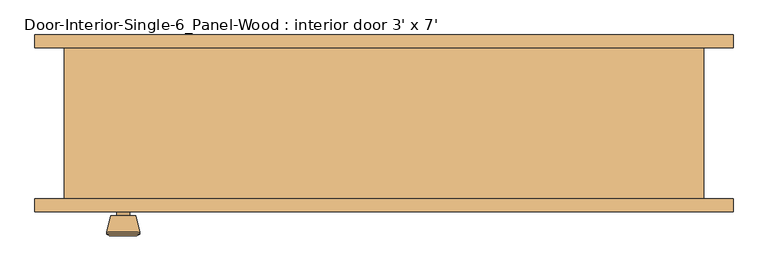
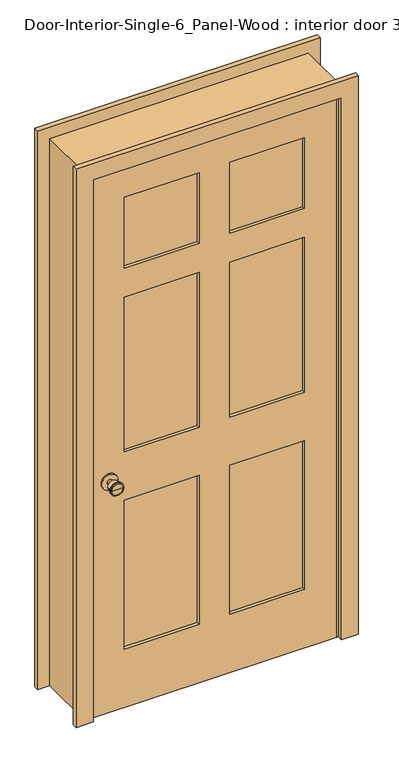
"""IFC4 building model written with IfcOpenShell, lengths in millimetres: door geometry, Door-Interior-Single-6_Panel-Wood : interior door 3' x 7'."""

from ifc_helpers import new_model, si_unit, point, frame, frame_2d, origin, place, context, project, spatial, polyline, circle_curve, trimmed, segment, composite_curve, outline, extrude, faceted_brep, source, transform, mapped, element, save
from ifc_brep_helpers import plane_surface, cylinder_surface, revolved_surface, advanced_brep


def door_interior_single_6_panel_wood_interior_door_3_x_7_c5239341(model_context):
    return source(origin(), model_context, "Body", "SolidModel", [
        advanced_brep(
        [(-393.7, -70.2, 914.4), (-403.7, -70.2, 914.4), (-383.7, -70.2, 914.4), (-373.2241324, -21.2, 914.4), (-414.1758676, -21.2, 914.4), (-393.7, -21.2, 914.4), (-368.7, -23.0278681, 914.4), (-418.7, -23.0278681, 914.4), (-368.7, -26.4915463, 914.4), (-418.7, -26.4915463, 914.4), (-375.063764, -51.2, 914.4), (-412.336236, -51.2, 914.4), (-383.7, -51.2, 914.4), (-403.7, -51.2, 914.4)],
        [
            (0, 1),
            (1, 2, circle_curve(frame((-393.7, -70.2, 914.4), z_axis=(0.0, -1.0, 0.0), x_axis=(-1.0, 0.0, 0.0)), 10.0)),
            (2, 0),
            (2, 1, circle_curve(frame((-393.7, -70.2, 914.4), z_axis=(0.0, -1.0, 0.0), x_axis=(-1.0, 0.0, 0.0)), 10.0)),
            (3, 4, circle_curve(frame((-393.7, -21.2, 914.4), z_axis=(0.0, 1.0, 0.0), x_axis=(-1.0, 0.0, 0.0)), 20.4758676)),
            (4, 5),
            (5, 3),
            (4, 3, circle_curve(frame((-393.7, -21.2, 914.4), z_axis=(0.0, 1.0, 0.0), x_axis=(-1.0, 0.0, 0.0)), 20.4758676)),
            (6, 7, circle_curve(frame((-393.7, -23.0278681, 914.4), z_axis=(0.0, 1.0, 0.0), x_axis=(-1.0, 0.0, 0.0)), 25.0)),
            (7, 4),
            (3, 6),
            (7, 6, circle_curve(frame((-393.7, -23.0278681, 914.4), z_axis=(0.0, 1.0, 0.0), x_axis=(-1.0, 0.0, 0.0)), 25.0)),
            (8, 9, circle_curve(frame((-393.7, -26.4915463, 914.4), z_axis=(0.0, 1.0, 0.0), x_axis=(-1.0, 0.0, 0.0)), 25.0)),
            (9, 7),
            (6, 8),
            (9, 8, circle_curve(frame((-393.7, -26.4915463, 914.4), z_axis=(0.0, 1.0, 0.0), x_axis=(-1.0, 0.0, 0.0)), 25.0)),
            (10, 11, circle_curve(frame((-393.7, -51.2, 914.4), z_axis=(0.0, 1.0, 0.0), x_axis=(-1.0, 0.0, 0.0)), 18.636236)),
            (11, 9),
            (8, 10),
            (11, 10, circle_curve(frame((-393.7, -51.2, 914.4), z_axis=(0.0, 1.0, 0.0), x_axis=(-1.0, 0.0, 0.0)), 18.636236)),
            (12, 13, circle_curve(frame((-393.7, -51.2, 914.4), z_axis=(0.0, 1.0, 0.0), x_axis=(-1.0, 0.0, 0.0)), 10.0)),
            (13, 11),
            (10, 12),
            (13, 12, circle_curve(frame((-393.7, -51.2, 914.4), z_axis=(0.0, 1.0, 0.0), x_axis=(-1.0, 0.0, 0.0)), 10.0)),
            (1, 13),
            (12, 2),
        ],
        [
            plane_surface(frame((-393.7, -70.2, 914.4), z_axis=(0.0, -1.0, 0.0), x_axis=(-1.0, 0.0, 0.0))),
            plane_surface(frame((-393.7, -21.2, 914.4), z_axis=(0.0, 1.0, 0.0), x_axis=(-1.0, 0.0, 0.0))),
            revolved_surface(polyline([(-414.1758676, -21.2, 914.4), (-418.7, -23.0278681, 914.4)]), (-393.7, -70.2, 914.4), (0.0, -1.0, 0.0)),
            cylinder_surface(frame((-393.7, -70.2, 914.4), z_axis=(0.0, -1.0, 0.0), x_axis=(-1.0, 0.0, 0.0)), 25.0),
            revolved_surface(polyline([(-418.7, -26.4915463, 914.4), (-412.336236, -51.2, 914.4)]), (-393.7, -70.2, 914.4), (0.0, -1.0, 0.0)),
            plane_surface(frame((-393.7, -51.2, 914.4), z_axis=(0.0, -1.0, 0.0), x_axis=(-1.0, 0.0, 0.0))),
            cylinder_surface(frame((-393.7, -70.2, 914.4), z_axis=(0.0, -1.0, 0.0), x_axis=(-1.0, 0.0, 0.0)), 10.0),
        ],
        [
            (0, [[1, 2, 3]]),
            (0, [[-3, 4, -1]]),
            (1, [[5, 6, 7]]),
            (1, [[8, -7, -6]]),
            (2, [[9, 10, -5, 11]]),
            (2, [[12, -11, -8, -10]]),
            (3, [[13, 14, -9, 15]]),
            (3, [[16, -15, -12, -14]]),
            (4, [[17, 18, -13, 19]]),
            (4, [[20, -19, -16, -18]]),
            (5, [[21, 22, -17, 23]]),
            (5, [[24, -23, -20, -22]]),
            (6, [[-2, 25, -21, 26]]),
            (6, [[-4, -26, -24, -25]]),
        ],
    ),
        extrude(outline(composite_curve([segment(trimmed(circle_curve(frame_2d((914.4, -393.7)), 30.0), [point((914.4, -423.7))], [point((914.4, -363.7))], False, "CARTESIAN"), True, "CONTINUOUS"), segment(trimmed(circle_curve(frame_2d((914.4, -393.7)), 30.0), [point((914.4, -363.7))], [point((914.4, -423.7))], False, "CARTESIAN"), True, "CONTINUOUS")], self_intersect=False)), frame((0.0, -76.2, 0.0), z_axis=(0.0, 1.0, 0.0), x_axis=(0.0, 0.0, 1.0)), (0.0, 0.0, 1.0), 6.0),
        advanced_brep(
        [(-393.7, -117.125, 914.4), (-383.7, -117.125, 914.4), (-403.7, -117.125, 914.4), (-373.2241324, -166.125, 914.4), (-393.7, -166.125, 914.4), (-414.1758676, -166.125, 914.4), (-368.7, -164.2971319, 914.4), (-418.7, -164.2971319, 914.4), (-368.7, -160.8334537, 914.4), (-418.7, -160.8334537, 914.4), (-375.063764, -136.125, 914.4), (-412.336236, -136.125, 914.4), (-383.7, -136.125, 914.4), (-403.7, -136.125, 914.4)],
        [
            (0, 1),
            (1, 2, circle_curve(frame((-393.7, -117.125, 914.4), z_axis=(0.0, 1.0, 0.0), x_axis=(-1.0, 0.0, 0.0)), 10.0)),
            (2, 0),
            (2, 1, circle_curve(frame((-393.7, -117.125, 914.4), z_axis=(0.0, 1.0, 0.0), x_axis=(-1.0, 0.0, 0.0)), 10.0)),
            (3, 4),
            (4, 5),
            (5, 3, circle_curve(frame((-393.7, -166.125, 914.4), z_axis=(0.0, -1.0, 0.0), x_axis=(-1.0, 0.0, 0.0)), 20.4758676)),
            (3, 5, circle_curve(frame((-393.7, -166.125, 914.4), z_axis=(0.0, -1.0, 0.0), x_axis=(-1.0, 0.0, 0.0)), 20.4758676)),
            (6, 3),
            (5, 7),
            (7, 6, circle_curve(frame((-393.7, -164.2971319, 914.4), z_axis=(0.0, -1.0, 0.0), x_axis=(-1.0, 0.0, 0.0)), 25.0)),
            (6, 7, circle_curve(frame((-393.7, -164.2971319, 914.4), z_axis=(0.0, -1.0, 0.0), x_axis=(-1.0, 0.0, 0.0)), 25.0)),
            (8, 6),
            (7, 9),
            (9, 8, circle_curve(frame((-393.7, -160.8334537, 914.4), z_axis=(0.0, -1.0, 0.0), x_axis=(-1.0, 0.0, 0.0)), 25.0)),
            (8, 9, circle_curve(frame((-393.7, -160.8334537, 914.4), z_axis=(0.0, -1.0, 0.0), x_axis=(-1.0, 0.0, 0.0)), 25.0)),
            (10, 8),
            (9, 11),
            (11, 10, circle_curve(frame((-393.7, -136.125, 914.4), z_axis=(0.0, -1.0, 0.0), x_axis=(-1.0, 0.0, 0.0)), 18.636236)),
            (10, 11, circle_curve(frame((-393.7, -136.125, 914.4), z_axis=(0.0, -1.0, 0.0), x_axis=(-1.0, 0.0, 0.0)), 18.636236)),
            (12, 10),
            (11, 13),
            (13, 12, circle_curve(frame((-393.7, -136.125, 914.4), z_axis=(0.0, -1.0, 0.0), x_axis=(-1.0, 0.0, 0.0)), 10.0)),
            (12, 13, circle_curve(frame((-393.7, -136.125, 914.4), z_axis=(0.0, -1.0, 0.0), x_axis=(-1.0, 0.0, 0.0)), 10.0)),
            (1, 12),
            (13, 2),
        ],
        [
            plane_surface(frame((-393.7, -117.125, 914.4), z_axis=(0.0, 1.0, 0.0), x_axis=(-1.0, 0.0, 0.0))),
            plane_surface(frame((-393.7, -166.125, 914.4), z_axis=(0.0, -1.0, 0.0), x_axis=(-1.0, 0.0, 0.0))),
            revolved_surface(polyline([(-414.1758676, -166.125, 914.4), (-418.7, -164.2971319, 914.4)]), (-393.7, -117.125, 914.4), (0.0, 1.0, 0.0)),
            cylinder_surface(frame((-393.7, -117.125, 914.4), z_axis=(0.0, 1.0, 0.0), x_axis=(-1.0, 0.0, 0.0)), 25.0),
            revolved_surface(polyline([(-418.7, -160.8334537, 914.4), (-412.336236, -136.125, 914.4)]), (-393.7, -117.125, 914.4), (0.0, 1.0, 0.0)),
            plane_surface(frame((-393.7, -136.125, 914.4), z_axis=(0.0, 1.0, 0.0), x_axis=(-1.0, 0.0, 0.0))),
            cylinder_surface(frame((-393.7, -117.125, 914.4), z_axis=(0.0, 1.0, 0.0), x_axis=(-1.0, 0.0, 0.0)), 10.0),
        ],
        [
            (0, [[1, 2, 3]]),
            (0, [[-3, 4, -1]]),
            (1, [[5, 6, 7]]),
            (1, [[-6, -5, 8]]),
            (2, [[9, -7, 10, 11]]),
            (2, [[-10, -8, -9, 12]]),
            (3, [[13, -11, 14, 15]]),
            (3, [[-14, -12, -13, 16]]),
            (4, [[17, -15, 18, 19]]),
            (4, [[-18, -16, -17, 20]]),
            (5, [[21, -19, 22, 23]]),
            (5, [[-22, -20, -21, 24]]),
            (6, [[25, -23, 26, -2]]),
            (6, [[-26, -24, -25, -4]]),
        ],
    ),
        extrude(outline(composite_curve([segment(trimmed(circle_curve(frame_2d((914.4, -393.7)), 30.0), [point((914.4, -423.7))], [point((914.4, -363.7))], False, "CARTESIAN"), True, "CONTINUOUS"), segment(trimmed(circle_curve(frame_2d((914.4, -393.7)), 30.0), [point((914.4, -363.7))], [point((914.4, -423.7))], False, "CARTESIAN"), True, "CONTINUOUS")], self_intersect=False)), frame((0.0, -117.125, 0.0), z_axis=(0.0, 1.0, 0.0), x_axis=(0.0, 0.0, 1.0)), (0.0, 0.0, 1.0), 6.0),
        faceted_brep([(482.6, -111.125, 0.0), (457.2, -111.125, 0.0), (457.2, -76.2, 0.0), (444.5, -76.2, 0.0), (444.5, -41.275, 0.0), (457.2, -41.275, 0.0), (457.2, 117.475, 0.0), (482.6, 117.475, 0.0), (482.6, 117.475, 2159.0), (482.6, -111.125, 2159.0), (457.2, 117.475, 2133.6), (-457.2, 117.475, 2133.6), (-457.2, 117.475, 0.0), (-482.6, 117.475, 0.0), (-482.6, 117.475, 2159.0), (457.2, -41.275, 2133.6), (444.5, -41.275, 2120.9), (-444.5, -41.275, 2120.9), (-444.5, -41.275, 0.0), (-457.2, -41.275, 0.0), (-457.2, -41.275, 2133.6), (444.5, -76.2, 2120.9), (457.2, -76.2, 2133.6), (-457.2, -76.2, 2133.6), (-457.2, -76.2, 0.0), (-444.5, -76.2, 0.0), (-444.5, -76.2, 2120.9), (457.2, -111.125, 2133.6), (-482.6, -111.125, 2159.0), (-482.6, -111.125, 0.0), (-457.2, -111.125, 0.0), (-457.2, -111.125, 2133.6)], [[[0, 1, 2, 3, 4, 5, 6, 7]], [[7, 8, 9, 0]], [[6, 10, 11, 12, 13, 14, 8, 7]], [[5, 15, 10, 6]], [[4, 16, 17, 18, 19, 20, 15, 5]], [[3, 21, 16, 4]], [[2, 22, 23, 24, 25, 26, 21, 3]], [[1, 27, 22, 2]], [[0, 9, 28, 29, 30, 31, 27, 1]], [[8, 14, 28, 9]], [[15, 20, 11, 10]], [[21, 26, 17, 16]], [[27, 31, 23, 22]], [[29, 13, 12, 19, 18, 25, 24, 30]], [[14, 13, 29, 28]], [[20, 19, 12, 11]], [[26, 25, 18, 17]], [[31, 30, 24, 23]]]),
        extrude(outline(polyline([(2133.6, -457.2), (0.0, -457.2), (0.0, 457.2), (2133.6, 457.2), (2133.6, -457.2)]), holes=[polyline([(2014.5375, 57.15), (2014.5375, 336.55), (1735.1375, 336.55), (1735.1375, 57.15), (2014.5375, 57.15)]), polyline([(1620.8375, 336.55), (1009.65, 336.55), (1009.65, 57.15), (1620.8375, 57.15), (1620.8375, 336.55)]), polyline([(1009.65, -57.15), (1009.65, -336.55), (1620.8375, -336.55), (1620.8375, -57.15), (1009.65, -57.15)]), polyline([(1735.1375, -336.55), (2014.5375, -336.55), (2014.5375, -57.15), (1735.1375, -57.15), (1735.1375, -336.55)]), polyline([(819.15, 57.15), (819.15, 336.55), (231.775, 336.55), (231.775, 57.15), (819.15, 57.15)]), polyline([(231.775, -57.15), (231.775, -336.55), (819.15, -336.55), (819.15, -57.15), (231.775, -57.15)])]), frame((0.0, -111.125, 0.0), z_axis=(0.0, 1.0, 0.0), x_axis=(0.0, 0.0, 1.0)), (0.0, 0.0, 1.0), 34.925),
        extrude(outline(polyline([(336.55, -87.8416667), (336.55, -99.4833333), (57.15, -99.4833333), (57.15, -87.8416667), (336.55, -87.8416667)])), frame((0.0, 0.0, 1735.1375), z_axis=(0.0, 0.0, 1.0), x_axis=(1.0, 0.0, 0.0)), (0.0, 0.0, 1.0), 279.4),
        extrude(outline(polyline([(336.55, -87.8416667), (336.55, -99.4833333), (57.15, -99.4833333), (57.15, -87.8416667), (336.55, -87.8416667)])), frame((0.0, 0.0, 1009.65), z_axis=(0.0, 0.0, 1.0), x_axis=(1.0, 0.0, 0.0)), (0.0, 0.0, 1.0), 611.1875),
        extrude(outline(polyline([(-57.15, -87.8416667), (-57.15, -99.4833333), (-336.55, -99.4833333), (-336.55, -87.8416667), (-57.15, -87.8416667)])), frame((0.0, 0.0, 1009.65), z_axis=(0.0, 0.0, 1.0), x_axis=(1.0, 0.0, 0.0)), (0.0, 0.0, 1.0), 611.1875),
        extrude(outline(polyline([(-57.15, -87.8416667), (-57.15, -99.4833333), (-336.55, -99.4833333), (-336.55, -87.8416667), (-57.15, -87.8416667)])), frame((0.0, 0.0, 1735.1375), z_axis=(0.0, 0.0, 1.0), x_axis=(1.0, 0.0, 0.0)), (0.0, 0.0, 1.0), 279.4),
        extrude(outline(polyline([(336.55, -87.8416667), (336.55, -99.4833333), (57.15, -99.4833333), (57.15, -87.8416667), (336.55, -87.8416667)])), frame((0.0, 0.0, 231.775), z_axis=(0.0, 0.0, 1.0), x_axis=(1.0, 0.0, 0.0)), (0.0, 0.0, 1.0), 587.375),
        extrude(outline(polyline([(-57.15, -87.8416667), (-57.15, -99.4833333), (-336.55, -99.4833333), (-336.55, -87.8416667), (-57.15, -87.8416667)])), frame((0.0, 0.0, 231.775), z_axis=(0.0, 0.0, 1.0), x_axis=(1.0, 0.0, 0.0)), (0.0, 0.0, 1.0), 587.375),
        extrude(outline(polyline([(0.0, 527.05), (2203.45, 527.05), (2203.45, -527.05), (0.0, -527.05), (0.0, -463.55), (2139.95, -463.55), (2139.95, 463.55), (0.0, 463.55), (0.0, 527.05)])), frame((0.0, -130.175, 0.0), z_axis=(0.0, 1.0, 0.0), x_axis=(0.0, 0.0, 1.0)), (0.0, 0.0, 1.0), 19.05),
        extrude(outline(polyline([(0.0, 527.05), (2203.45, 527.05), (2203.45, -527.05), (0.0, -527.05), (0.0, -463.55), (2139.95, -463.55), (2139.95, 463.55), (0.0, 463.55), (0.0, 527.05)])), frame((0.0, 117.475, 0.0), z_axis=(0.0, 1.0, 0.0), x_axis=(0.0, 0.0, 1.0)), (0.0, 0.0, 1.0), 19.05),
    ])


if __name__ == "__main__":
    model = new_model("IFC4")
    model_context = context("Model", 3, world=origin())
    ifc_project = project(units=[si_unit("LENGTHUNIT", "METRE", prefix="MILLI")], contexts=[model_context])
    site = spatial("IfcSite", under=ifc_project)
    building = spatial("IfcBuilding", under=site)
    placement = place(None, origin())
    door_interior_single_6_panel_wood_interior_door_3_x_7_shape = door_interior_single_6_panel_wood_interior_door_3_x_7_c5239341(model_context)
    element("IfcDoor", 1, ObjectType="Door-Interior-Single-6_Panel-Wood : interior door 3' x 7'", at=placement, inside=building, context=model_context, shape_type="MappedRepresentation", body=[
        mapped(door_interior_single_6_panel_wood_interior_door_3_x_7_shape, transform((0.0, 0.0, 0.0), x_axis=(1.0, 0.0, 0.0), y_axis=(0.0, 1.0, 0.0), z_axis=(0.0, 0.0, 1.0))),
    ])
    save(model, "model.ifc")

# Revit data of these elements
# Type "Door-Interior-Single-6_Panel-Wood : interior door 3' x 7'"
#   Type Mark = "13"
#   Assembly Code = "C1020300"
#   Analytic Construction = "Wooden"
#   Top Rail = 0' - 4 11/16"
#   Top Panel = 0' - 11"
#   Thickness = 0' - 1 3/8"
#   Thermal Resistance (R) = 2.5876 (h·ft²·°F)/BTU
#   Swing Angle [instance default] = 90.00°
#   Stiles = 0' - 4 3/4"
#   Rough Width = 3' - 2"
#   Rough Height = 7' - 1"
#   Mullion = 0' - 4 1/2"
#   Lock Rail = 0' - 7 1/2"
#   Intermediate Rail = 0' - 4 1/2"
#   Height = 7' - 0"
#   Width = 3' - 0"
#   Heat Transfer Coefficient (U) = 0.3865 BTU/(h·ft²·°F)
#   Bottom Rail = 0' - 9 1/8"
#   Trim Material = Cherry
#   Panel Material = Cherry
#   Frame Material = Cherry
#   Door Handle Material = Aluminum
#   Visual Light Transmittance = 0
#   Solar Heat Gain Coefficient = 0
#   Wall Closure = (empty or 0)
#   Function = (empty or 0)
# Element 1 (IfcDoor, "Door-Interior-Single-6_Panel-Wood : interior door 3' x 7'")
#   Materials on its faces: "Cherry", "Aluminum"
# Materials
#   "Cherry": class "Wood", colour RGB 226 177 128, transparency 0, Description = "Prunus Serotina", Cost = 0
#   "Aluminum": class "Metal", colour RGB 247 247 247, transparency 0, Description = "Aluminum 6061", Cost = 0
